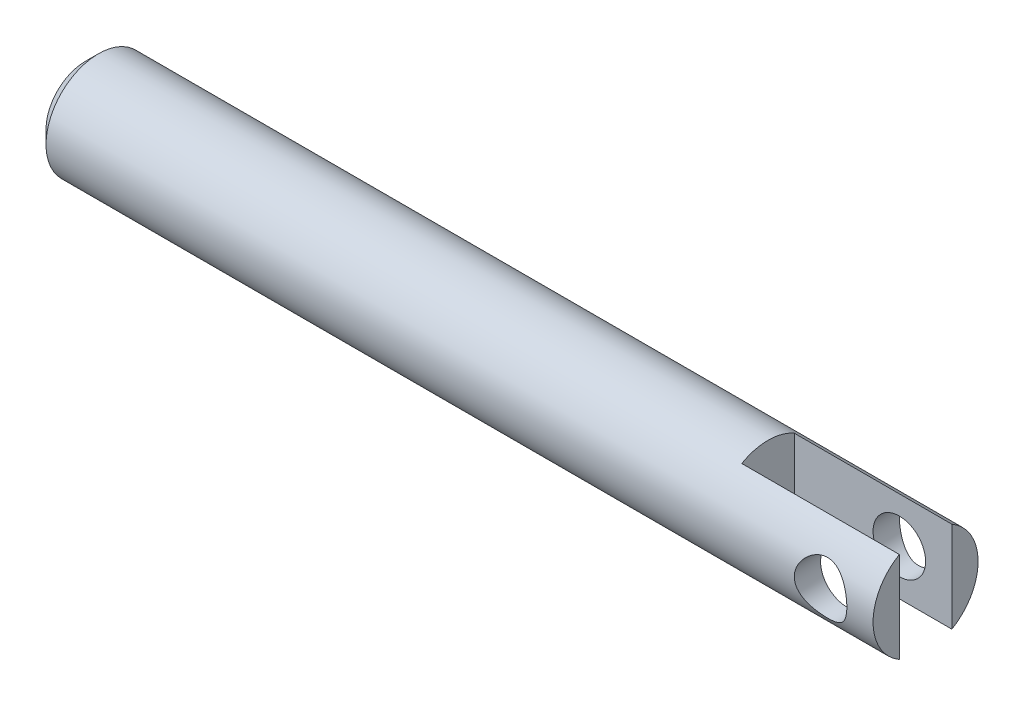
SolidWorks part; units mm, degrees
material "Plain Carbon Steel"
ref_plane "Front Plane" through (0, 0, 0) normal (0, 0, 1) x (1, 0, 0)
ref_plane "Top Plane" through (0, 0, 0) normal (0, 1, 0) x (1, 0, 0)
ref_plane "Right Plane" through (0, 0, 0) normal (1, 0, 0) x (0, 0, -1)
sketch "Rod Profile Sketch" plane through (0, 0, 0) normal (0, 0, 1) x (1, 0, 0)
  line L0 (-2.2934, 0) -> (1.5428, 0) construction
  line L2 (-2, 0.25) -> (2, 0.25)
  line L3 (-2, 0.25) -> (-2, 0)
  line L4 (-2, 0) -> (2, 0)
  line L5 (2, 0.25) -> (2, 0)
  dimension "D1" = 0.25
  dimension "D2" = 4
  dimension "D3" = 2
revolve "Rod Body" add sketch "Rod Profile Sketch" angle 360 about L0
sketch "End Notch Sketch" plane through (0, 0, 0) normal (0, 0, 1) x (1, 0, 0)
  line L0 (0, 0) -> (2.5009, 0) construction
  line L1 (2, -0.25) -> (2, 0.25) construction
  circle A0 centre (1.75, 0) radius 0.125
  dimension "D2" = 0.25
  dimension "D1" = 0.25
extrude "End Notch Cut" cut sketch "End Notch Sketch" against normal mid plane 10
sketch "Clevis Slot Sketch" plane through (0, 0, 0) normal (0, 1, 0) x (1, 0, 0)
  line L0 (0, 0) -> (2.3489, 0) construction
  line L1 (2, -0.25) -> (2, 0.25) construction
  line L2 (1.25, -0.125) -> (2, -0.125)
  line L3 (1.25, -0.125) -> (1.25, 0.125)
  line L4 (1.25, 0.125) -> (2, 0.125)
  line L5 (2, -0.125) -> (2, 0.125)
  line L6 (1.25, -0.125) -> (2, 0.125) construction
  line L7 (1.25, 0.125) -> (2, -0.125) construction
  point P3 (1.625, 0)
  dimension "D1" = 0.25
  dimension "D2" = 0.75
extrude "Clevis Slot" cut sketch "Clevis Slot Sketch" against normal mid plane 10
sketch "Cross Pin Hole Sketch" plane through (-2, 0, 0) normal (-1, 0, 0) x (0, 0, 1)
  circle A0 centre (0, 0) radius 0.1562
  dimension "D1" = 0.3125
extrude "Cross Pin Hole" cut sketch "Cross Pin Hole Sketch" against normal blind 1.75
chamfer "End Chamfer" distance 0.0625 angle 45 1 edges at (-2, 0, 0.25)
scale "Scale to Final Size" scale about origin uniform scaling yes scale factor 25.4
